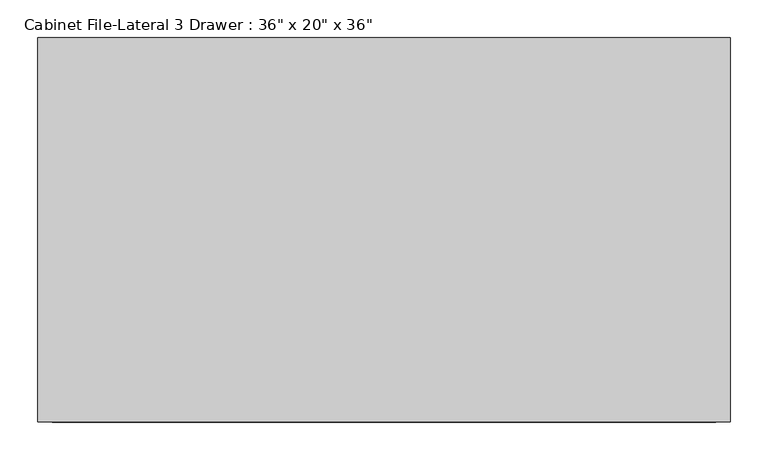
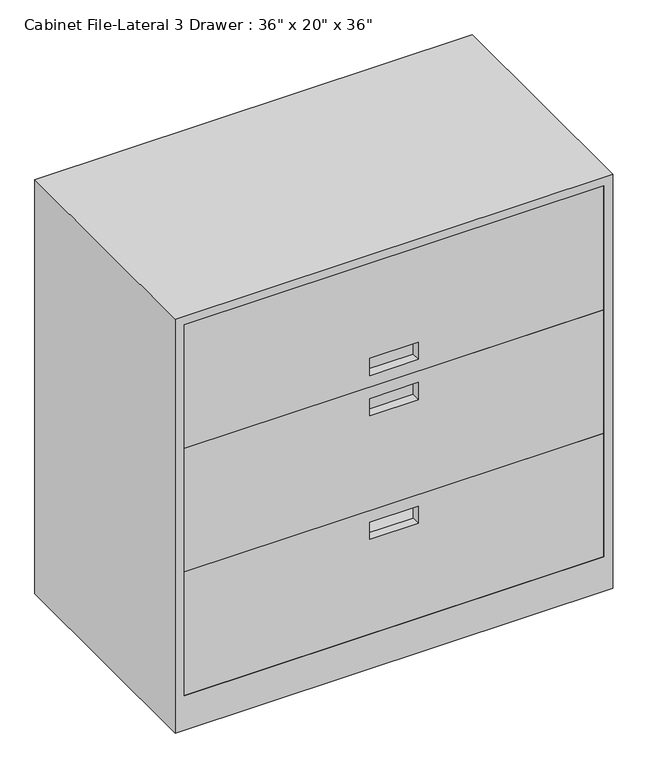
"""IFC4 building model written with IfcOpenShell, lengths in millimetres: furniture geometry."""

from ifc_helpers import new_model, si_unit, frame, origin, place, context, project, spatial, polyline, outline, extrude, faceted_brep, source, transform, mapped, element, save


def furniture_dccb195e(model_context):
    return source(origin(), model_context, "Body", "SolidModel", [
        faceted_brep([(277.1774861, -680.3183761, 914.4), (-637.2225139, -680.3183761, 914.4), (-637.2225139, -1188.3183761, 914.4), (277.1774861, -1188.3183761, 914.4), (277.1774861, -680.3183761, 0.0), (277.1774861, -1188.3183761, 0.0), (-637.2225139, -1188.3183761, 0.0), (-637.2225139, -680.3183761, 0.0), (258.1274861, -1188.3183761, 76.2), (-618.1725139, -1188.3183761, 76.2), (-618.1725139, -1188.3183761, 895.35), (258.1274861, -1188.3183761, 895.35), (-618.1725139, -699.3683761, 76.2), (258.1274861, -699.3683761, 76.2), (258.1274861, -699.3683761, 895.35), (-618.1725139, -699.3683761, 895.35)], [[[0, 1, 2, 3]], [[4, 5, 6, 7]], [[1, 0, 4, 7]], [[2, 1, 7, 6]], [[3, 2, 6, 5], [8, 9, 10, 11]], [[0, 3, 5, 4]], [[12, 13, 14, 15]], [[13, 12, 9, 8]], [[14, 13, 8, 11]], [[15, 14, 11, 10]], [[12, 15, 10, 9]]]),
        extrude(outline(polyline([(895.35, -618.1725139), (622.2999998, -618.1725139), (622.3, 258.1274861), (895.35, 258.1274861), (895.35, -618.1725139)]), holes=[polyline([(685.8, -230.8225139), (685.8, -129.2225139), (647.7, -129.2225139), (647.7, -230.8225139), (685.8, -230.8225139)])]), frame((0.0, -1188.3183761, 0.0), z_axis=(0.0, 1.0, 0.0), x_axis=(0.0, 0.0, 1.0)), (0.0, 0.0, 1.0), 19.05),
        extrude(outline(polyline([(349.25, -618.1725139), (349.25, 258.1274861), (622.3, 258.1274861), (622.2999998, -618.1725139), (349.25, -618.1725139)]), holes=[polyline([(596.9, -230.8225139), (596.9, -129.2225139), (558.8, -129.2225139), (558.8, -230.8225139), (596.9, -230.8225139)])]), frame((0.0, -1188.3183761, 0.0), z_axis=(0.0, 1.0, 0.0), x_axis=(0.0, 0.0, 1.0)), (0.0, 0.0, 1.0), 19.05),
        extrude(outline(polyline([(76.2, -618.1725139), (76.2, 258.1274861), (349.25, 258.1274861), (349.25, -618.1725139), (76.2, -618.1725139)]), holes=[polyline([(323.85, -230.8225139), (323.85, -129.2225139), (285.75, -129.2225139), (285.75, -230.8225139), (323.85, -230.8225139)])]), frame((0.0, -1188.3183761, 0.0), z_axis=(0.0, 1.0, 0.0), x_axis=(0.0, 0.0, 1.0)), (0.0, 0.0, 1.0), 19.05),
    ])


if __name__ == "__main__":
    model = new_model("IFC4")
    model_context = context("Model", 3, world=origin())
    ifc_project = project(units=[si_unit("LENGTHUNIT", "METRE", prefix="MILLI")], contexts=[model_context])
    site = spatial("IfcSite", under=ifc_project)
    building = spatial("IfcBuilding", under=site)
    placement = place(None, origin())
    furniture_shape = furniture_dccb195e(model_context)
    element("IfcFurniture", 1, ObjectType="Cabinet File-Lateral 3 Drawer : 36\" x 20\" x 36\"", at=placement, inside=building, context=model_context, shape_type="MappedRepresentation", body=[
        mapped(furniture_shape, transform((0.0, 0.0, 0.0), x_axis=(1.0, 0.0, 0.0), y_axis=(0.0, 1.0, 0.0), z_axis=(0.0, 0.0, 1.0))),
    ])
    save(model, "model.ifc")

# Revit data of these elements
# Type "Cabinet File-Lateral 3 Drawer : 36\" x 20\" x 36\""
#   Assembly Code = "E2020200"
#   Depth = 1' - 8"
#   Height = 3' - 0"
#   Width = 3' - 0"
#   Material = Metal - Steel
#   Default Elevation = 0
# Element 1 (IfcFurniture, "Cabinet File-Lateral 3 Drawer : 36\" x 20\" x 36\"")
#   Materials on its faces: "Metal - Steel"
# Materials
#   "Metal - Steel": colour RGB 209 209 209, transparency 0
